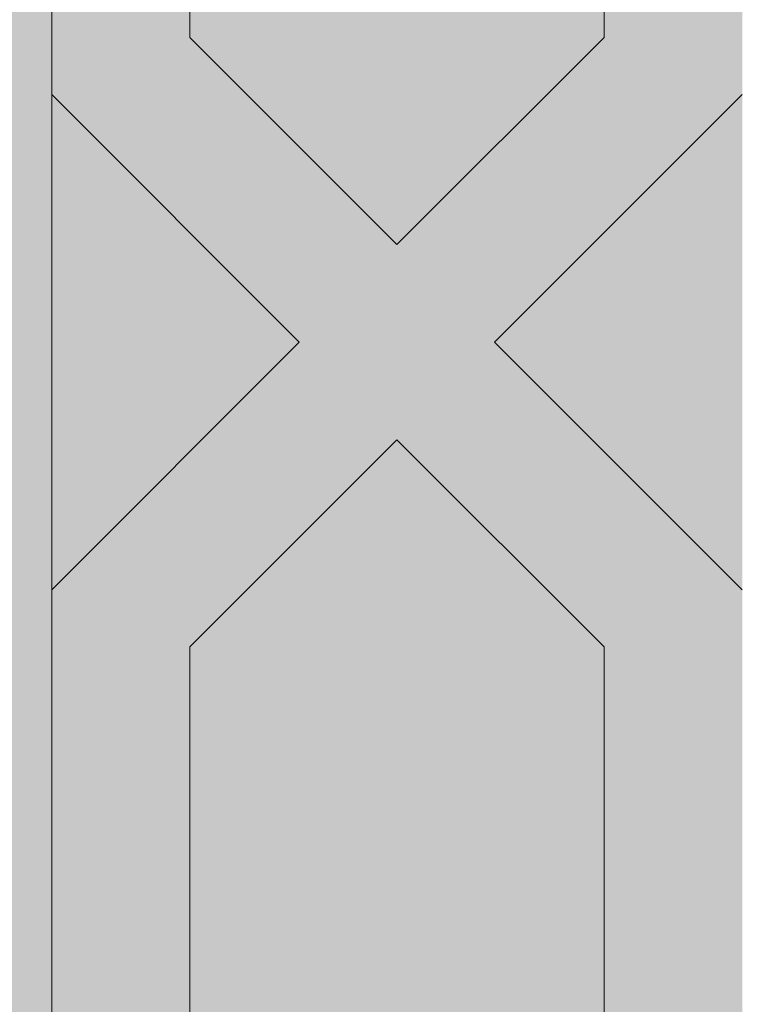
# Model space of a CAD drawing. Units: inches. Extents: x 844 to 2234, y 346 to 1084.
# Tile 17 of 93: x 1116.421 to 1117.756, y 703.242 to 705.06. Entities that reach past the tile are written whole.
import ezdxf

# ---------------------------------------------------------------- set-up
doc = ezdxf.new("R2010")
doc.units = ezdxf.units.IN
doc.header["$MEASUREMENT"] = 0
for name, color, linetype, lineweight in [('A-ANNO-DIMS', 2, 'Continuous', 18), ('furniture', 8, 'Continuous', 18), ('RA-AP-01$0$INT', 35, 'Continuous', 5)]:
    doc.layers.add(name, color=color, linetype=linetype, lineweight=lineweight)
doc.layers.add('RA-AP-01$0$FURN', color=3, linetype='Continuous')
doc.styles.get("Standard").update_dxf_attribs({"font": 'arial.ttf'})
doc.dimstyles.get("Standard").update_dxf_attribs({"dimtxt": 6, "dimasz": 3, "dimexe": 0.18, "dimexo": 0.0625, "dimgap": 0.09, "dimtad": 0, "dimtih": 1, "dimtoh": 1, "dimdec": 1, "dimzin": 0, "dimdsep": 46, "dimlunit": 3, "dimtxsty": 'Standard', "dimblk": 'ARCHTICK', "dimcen": 0.09, "dimadec": 0, "dimazin": 0, "dimtfac": 1, "dimtdec": 1, "dimtofl": 0, "dimtmove": 0, "dimatfit": 3, "dimfxl": 1, "dimtolj": 1, "dimtzin": 0, "dimarcsym": 0})

# ---------------------------------------------------------------- blocks, each defined once
blk = doc.blocks.new('A$C18D01794')
at = {"layer": 'RA-AP-01$0$INT'}
h = blk.add_hatch(color=256, dxfattribs=at)
h.paths.add_polyline_path([(4.355206456958071, -6.156712009588037), (4.355206456958071, -8.056712009588038), (5.455206456958072, -8.056712009588038), (5.455206456958072, -6.156712009588037)])
h.paths.add_polyline_path([(4.405206456958072, -8.006712009588039), (4.405206456958072, -6.206712009588038), (5.405206456958072, -6.206712009588038), (5.405206456958072, -8.006712009588039)], flags=16)
h = blk.add_hatch(color=256, dxfattribs=at)
h.paths.add_polyline_path([(4.505206456958071, -7.585498806127123), (4.46934859260189, -7.549640941759413), (4.505206456958071, -7.513783077414768), (4.505206456958071, -7.381963272220687), (4.469348592616735, -7.346105407867824), (4.505206456958071, -7.310247543514964), (4.505206456958071, -7.178427738324996), (4.469348592586679, -7.142569873965138), (4.505206456952245, -7.106712009588038), (4.476922185709333, -7.106712009588038), (4.455206456960671, -7.128427738343681), (4.433490728198047, -7.106712009588038), (4.405206456946033, -7.106712009588036), (4.441064321339216, -7.142569873969684), (4.40520645695807, -7.178427738362358), (4.405206456958072, -7.310247543472698), (4.441064321364728, -7.346105407867826), (4.40520645695807, -7.381963272262947), (4.40520645695807, -7.513783077378263), (4.441064321354429, -7.549640941786153), (4.405206456958072, -7.585498806170974), (4.405206456958072, -7.717318611286652), (4.441064321333084, -7.753176475673194), (4.405206456958072, -7.789034340036673), (4.405206456958072, -8.006712009588039), (4.644348592588106, -8.006712009588039), (4.680206456964639, -7.970854145211967), (4.716064321341165, -8.006712009588039), (4.869348592586113, -8.006712009588039), (4.905206456964143, -7.970854145210465), (4.941064321342174, -8.006712009588039), (5.094348592587118, -8.006712009588037), (5.130206456963649, -7.970854145211967), (5.166064321340178, -8.006712009588039), (5.405206456958072, -8.006712009588039), (5.405206456958072, -7.789034340024526), (5.369348592595202, -7.753176475673196), (5.40520645695807, -7.717318611298797), (5.40520645695807, -7.585498806158829), (5.369348592573859, -7.549640941786151), (5.40520645695807, -7.51378307739041), (5.40520645695807, -7.381963272250803), (5.36934859256356, -7.346105407867824), (5.405206456958072, -7.310247543484846), (5.405206456958072, -7.178427738350217), (5.369348592589068, -7.142569873969682), (5.405206456982249, -7.106712009588038), (5.376922185730244, -7.106712009588038), (5.355206456967613, -7.128427738343679), (5.333490728218955, -7.10671200958804), (5.305206456976043, -7.106712009588042), (5.341064321341609, -7.142569873965136), (5.305206456958072, -7.178427738337141), (5.305206456958072, -7.310247543502816), (5.34106432131155, -7.346105407867824), (5.305206456958072, -7.381963272232832), (5.30520645695807, -7.513783077402624), (5.341064321326395, -7.549640941759413), (5.305206456958072, -7.585498806139263), (5.305206456958072, -7.717318611299605), (5.341064321347738, -7.753176475677737), (5.305206456958072, -7.78903434007894), (5.30520645695807, -7.906712009588039), (5.166064321336834, -7.906712009588039), (5.130206456963647, -7.942569873961684), (5.094348592590464, -7.906712009588039), (4.941064321338827, -7.906712009588041), (4.905206456964145, -7.942569873963183), (4.869348592589459, -7.906712009588039), (4.716064321337822, -7.906712009588041), (4.680206456964641, -7.942569873961684), (4.644348592591453, -7.906712009588039), (4.505206456958071, -7.906712009588039), (4.505206456958071, -7.789034340066795), (4.469348592580545, -7.753176475677738), (4.505206456958071, -7.717318611311748)])
h.paths.add_polyline_path([(4.485206456974132, -7.709034340046354), (4.45520645695909, -7.739034340051736), (4.425206456974128, -7.709034340057131), (4.425206456993394, -7.593783077384998), (4.45520645699153, -7.563783077396511), (4.485206456993396, -7.593783077408017)], flags=16)
h.paths.add_polyline_path([(4.455206456954537, -7.767318611299197), (4.485206456958242, -7.797318611312542), (4.48520645695951, -7.912569873958716), (4.45520645695415, -7.942569873954422), (4.425206456957888, -7.912569873967813), (4.425206456957888, -7.797318611286197)], flags=16)
h.paths.add_polyline_path([(4.455206456964794, -7.535498806149051), (4.42520645696469, -7.5054988061393), (4.425206456983954, -7.390247543486406), (4.455206456990734, -7.360247543489279), (4.485206456983953, -7.39024754349214), (4.485206456964687, -7.505498806158811)], flags=16)
h.paths.add_polyline_path([(4.499348592588947, -7.926712009585049), (4.636064321340932, -7.926712009585049), (4.666064321342317, -7.956712009586821), (4.636064321343707, -7.986712009585048), (4.499348592575121, -7.986712009585048), (4.469348592591685, -7.956712009591957)], flags=16)
h.paths.add_polyline_path([(4.425206456957888, -7.940854145195974), (4.471064321332215, -7.986712009585049), (4.425206456957888, -7.986712009585049)], flags=16)
h.paths.add_polyline_path([(4.455206456990734, -7.331963272246367), (4.425206456989053, -7.301963272254337), (4.425206456969784, -7.186712009596224), (4.455206456965226, -7.156712009591144), (4.485206456969787, -7.186712009586051), (4.485206456989053, -7.301963272238404)], flags=16)
h.paths.add_polyline_path([(4.72434859258714, -7.926712009586255), (4.861064321340141, -7.926712009586248), (4.891064321340324, -7.956712009586823), (4.861064321340513, -7.986712009586252), (4.724348592586768, -7.986712009586252), (4.694348592586956, -7.956712009586821)], flags=16)
h.paths.add_polyline_path([(4.919348592587961, -7.956712009586821), (4.949348592588145, -7.92671200958625), (5.08606432134115, -7.926712009586253), (5.116064321341327, -7.956712009586823), (5.086064321341519, -7.986712009586252), (4.949348592587774, -7.986712009586252)], flags=16)
h.paths.add_polyline_path([(5.144348592585967, -7.956712009586823), (5.174348592587358, -7.926712009585049), (5.311064321339338, -7.926712009585049), (5.3410643213366, -7.956712009591957), (5.311064321353163, -7.986712009585048), (5.174348592584576, -7.986712009585048)], flags=16)
h.paths.add_polyline_path([(5.32520645693489, -7.593783077408021), (5.355206456936755, -7.563783077396511), (5.385206456934894, -7.593783077384998), (5.38520645695416, -7.709034340057128), (5.355206456969194, -7.739034340051736), (5.325206456954153, -7.709034340046352)], flags=16)
h.paths.add_polyline_path([(5.325206456970042, -7.797318611312542), (5.355206456973747, -7.767318611299197), (5.385206456970398, -7.7973186112862), (5.385206456970398, -7.912569873967816), (5.355206456974136, -7.942569873954422), (5.325206456968778, -7.912569873958716)], flags=16)
h.paths.add_polyline_path([(5.325206456963599, -7.505498806158811), (5.325206456944333, -7.39024754349214), (5.355206456937552, -7.360247543489279), (5.385206456944332, -7.39024754348641), (5.385206456963596, -7.505498806139303), (5.355206456963492, -7.53549880614905)], flags=16)
h.paths.add_polyline_path([(5.32520645693923, -7.301963272238403), (5.3252064569585, -7.186712009586051), (5.355206456963062, -7.156712009591142), (5.3852064569585, -7.186712009596224), (5.385206456939234, -7.301963272254338), (5.355206456937552, -7.331963272246369)], flags=16)
h.paths.add_polyline_path([(5.339348592596071, -7.986712009585048), (5.385206456970398, -7.940854145195972), (5.385206456970396, -7.986712009585048)], flags=16)
h = blk.add_hatch(color=256, dxfattribs=at)
h.paths.add_polyline_path([(4.469348592586677, -7.142569873965136), (4.505206456958073, -7.178427738324996), (4.505206456958071, -7.106712009582215)])
h.paths.add_polyline_path([(4.455206456960671, -7.128427738343681), (4.476922185709333, -7.106712009588038), (4.433490728198045, -7.106712009588038)])
h.paths.add_polyline_path([(4.405206456958073, -7.178427738362358), (4.441064321339218, -7.142569873969684), (4.40520645695807, -7.106712009600073)])
h.paths.add_polyline_path([(4.425206456989053, -7.301963272254335), (4.455206456990736, -7.331963272246371), (4.485206456989055, -7.301963272238399), (4.48520645696979, -7.186712009586054), (4.455206456965227, -7.15671200959114), (4.425206456969784, -7.186712009596224)])
h.paths.add_polyline_path([(4.505206456958073, -7.381963272220689), (4.505206456958071, -7.310247543514961), (4.469348592616738, -7.346105407867826)])
h.paths.add_polyline_path([(4.425206456964688, -7.5054988061393), (4.455206456964794, -7.535498806149051), (4.485206456964689, -7.505498806158811), (4.485206456983951, -7.390247543492138), (4.455206456990736, -7.360247543489277), (4.425206456983956, -7.39024754348641)])
h.paths.add_polyline_path([(4.425206456974126, -7.709034340057128), (4.455206456959092, -7.739034340051736), (4.485206456974132, -7.709034340046356), (4.485206456993396, -7.593783077408017), (4.45520645699153, -7.563783077396511), (4.425206456993394, -7.593783077384999)])
h.paths.add_polyline_path([(4.46934859260189, -7.549640941759415), (4.505206456958071, -7.585498806127123), (4.505206456958073, -7.513783077414766)])
h.paths.add_polyline_path([(4.405206456958073, -7.585498806170972), (4.441064321354427, -7.549640941786151), (4.405206456958072, -7.513783077378263)])
h.paths.add_polyline_path([(4.405206456958072, -7.789034340036673), (4.441064321333084, -7.753176475673194), (4.405206456958072, -7.71731861128665)])
h.paths.add_polyline_path([(4.469348592580547, -7.75317647567774), (4.505206456958071, -7.789034340066795), (4.505206456958071, -7.717318611311744)])
h.paths.add_polyline_path([(4.425206456957888, -7.912569873967814), (4.45520645695415, -7.942569873954422), (4.485206456959507, -7.912569873958718), (4.48520645695824, -7.797318611312542), (4.455206456954537, -7.767318611299197), (4.425206456957888, -7.797318611286202)])
h.paths.add_polyline_path([(4.425206456957888, -7.986712009585049), (4.471064321332215, -7.986712009585049), (4.425206456957888, -7.940854145195972)])
h.paths.add_polyline_path([(4.499348592575121, -7.986712009585048), (4.636064321343707, -7.986712009585049), (4.666064321342317, -7.956712009586823), (4.636064321340932, -7.926712009585049), (4.499348592588945, -7.926712009585049), (4.469348592591685, -7.95671200959196)])
h.paths.add_polyline_path([(4.680206456964641, -7.942569873961684), (4.716064321337824, -7.906712009588039), (4.644348592591454, -7.906712009588039)])
h.paths.add_polyline_path([(4.644348592588108, -8.006712009588039), (4.716064321341167, -8.006712009588039), (4.680206456964637, -7.970854145211964)])
h.paths.add_polyline_path([(4.724348592586768, -7.98671200958625), (4.861064321340514, -7.986712009586252), (4.891064321340324, -7.956712009586819), (4.861064321340141, -7.92671200958625), (4.724348592587134, -7.926712009586255), (4.694348592586957, -7.956712009586821)])
h.paths.add_polyline_path([(4.905206456964143, -7.942569873963183), (4.941064321338827, -7.906712009588039), (4.869348592589457, -7.906712009588037)])
h.paths.add_polyline_path([(4.869348592586113, -8.006712009588039), (4.941064321342172, -8.006712009588037), (4.905206456964145, -7.970854145210463)])
h.paths.add_polyline_path([(4.949348592587774, -7.986712009586252), (5.086064321341521, -7.986712009586252), (5.116064321341329, -7.956712009586823), (5.08606432134115, -7.926712009586253), (4.949348592588145, -7.92671200958625), (4.919348592587961, -7.956712009586819)])
h.paths.add_polyline_path([(5.130206456963645, -7.942569873961684), (5.166064321336834, -7.906712009588039), (5.094348592590464, -7.906712009588039)])
h.paths.add_polyline_path([(5.094348592587119, -8.006712009588039), (5.166064321340178, -8.006712009588039), (5.130206456963651, -7.970854145211967)])
h.paths.add_polyline_path([(5.174348592584578, -7.986712009585048), (5.311064321353163, -7.986712009585048), (5.341064321336602, -7.956712009591958), (5.31106432133934, -7.926712009585049), (5.174348592587352, -7.926712009585049), (5.144348592585969, -7.956712009586823)])
h.paths.add_polyline_path([(5.325206456968778, -7.912569873958718), (5.355206456974136, -7.942569873954422), (5.385206456970396, -7.912569873967814), (5.385206456970396, -7.797318611286199), (5.355206456973747, -7.767318611299197), (5.325206456970044, -7.797318611312544)])
h.paths.add_polyline_path([(5.339348592596073, -7.986712009585048), (5.385206456970396, -7.986712009585049), (5.385206456970398, -7.94085414519597)])
h.paths.add_polyline_path([(5.325206456954155, -7.709034340046354), (5.355206456969194, -7.739034340051734), (5.38520645695416, -7.709034340057128), (5.385206456934896, -7.593783077384999), (5.355206456936758, -7.563783077396513), (5.325206456934888, -7.593783077408019)])
h.paths.add_polyline_path([(5.305206456958072, -7.789034340078938), (5.341064321347739, -7.753176475677738), (5.305206456958072, -7.717318611299605)])
h.paths.add_polyline_path([(5.369348592595204, -7.753176475673194), (5.40520645695807, -7.789034340024526), (5.405206456958072, -7.717318611298798)])
h.paths.add_polyline_path([(5.405206456958072, -7.585498806158831), (5.405206456958072, -7.513783077390407), (5.369348592573857, -7.549640941786151)])
h.paths.add_polyline_path([(5.305206456958072, -7.585498806139266), (5.341064321326393, -7.549640941759413), (5.305206456958072, -7.513783077402626)])
h.paths.add_polyline_path([(5.325206456963599, -7.50549880615881), (5.355206456963494, -7.535498806149055), (5.385206456963598, -7.505498806139302), (5.385206456944334, -7.390247543486411), (5.355206456937552, -7.360247543489279), (5.325206456944333, -7.39024754349214)])
h.paths.add_polyline_path([(5.305206456958072, -7.38196327223283), (5.341064321311551, -7.346105407867824), (5.305206456958072, -7.31024754350282)])
h.paths.add_polyline_path([(5.325206456939231, -7.301963272238404), (5.355206456937552, -7.331963272246369), (5.385206456939235, -7.301963272254335), (5.385206456958502, -7.186712009596224), (5.355206456963061, -7.156712009591142), (5.3252064569585, -7.186712009586051)])
h.paths.add_polyline_path([(5.404581768715993, -7.381338584008926, -0.001217816984214), (5.405206456958072, -7.381112009582329), (5.405206456958072, -7.310247543484846), (5.369348592563558, -7.346105407867826)])
h.paths.add_polyline_path([(5.36934859258907, -7.142569873969684), (5.40520645695807, -7.178427738350215), (5.405206456958072, -7.106712009612218)])
h.paths.add_polyline_path([(5.355206456967613, -7.128427738343683), (5.376922185730239, -7.106712009588038), (5.333490728218953, -7.10671200958804)])
h.paths.add_polyline_path([(5.30520645695807, -7.178427738337139), (5.341064321341609, -7.142569873965134), (5.305206456958074, -7.10671200957007)])
for p, q in [((4.425206456993394, -7.593783077384996), (4.425206456974128, -7.709034340057129)), ((4.485206456993396, -7.593783077408017), (4.485206456974132, -7.709034340046354)), ((4.425206456974128, -7.709034340057129), (4.455206456959092, -7.739034340051736)), ((4.485206456974132, -7.709034340046354), (4.455206456959092, -7.739034340051736)), ((4.405206456963013, -7.717318611291593), (4.441064321333084, -7.753176475673194)), ((4.505206456963013, -7.717318611306806), (4.469348592580547, -7.753176475677738)), ((4.441064321333084, -7.753176475673194), (4.405206456950156, -7.789034340044587)), ((4.469348592580547, -7.753176475677738), (4.505206456951941, -7.789034340060664)), ((4.455206456954537, -7.767318611299197), (4.425206456957888, -7.797318611286199)), ((4.455206456954537, -7.767318611299197), (4.485206456958242, -7.797318611312544)), ((4.425206456957888, -7.797318611286199), (4.425206456957888, -7.912569873967814)), ((4.485206456959509, -7.912569873958718), (4.485206456958242, -7.797318611312544))]:
    blk.add_line(p, q, dxfattribs=at)
blk.add_lwpolyline([(5.405206456958072, -8.006712009588039), (4.405206456958072, -8.006712009588039), (4.405206456958072, -7.106712009588038)], dxfattribs=at)
blk = doc.blocks.new('A$C5D2F253E')
at = {"layer": 'RA-AP-01$0$FURN', "xscale": -0.7999999999883585, "yscale": 0.7999999999883585, "zscale": 0.8, "rotation": 90}
blk.add_blockref('A$C18D01794', (-5.687757199772477, 4.75791982714071), dxfattribs=at)
blk = doc.blocks.new('_ArchTick')
at = {"color": 0, "linetype": 'ByBlock', "const_width": 0.15}
blk.add_lwpolyline([(-0.5, -0.5), (0.5, 0.5)], dxfattribs=at)
blk = doc.blocks.new('*D144')
at = {"layer": 'A-ANNO-DIMS', "color": 0, "lineweight": -2, "transparency": 16777216}
for p, q in [((1096.615948, 439.3732739999999), (1096.615948, 1074.743301)), ((1143.115948, 492.373274), (1143.115948, 1074.743301)), ((1096.615948, 1074.563301), (1102.481950728513, 1074.563301)), ((1143.115948, 1074.563301), (1137.249945271487, 1074.563301))]:
    blk.add_line(p, q, dxfattribs=at)
at = {"layer": 'Defpoints', "color": 0, "transparency": 16777216}
for p in [(1143.115948, 1074.563301), (1143.115948, 492.3107739999999), (1096.615948, 439.3107739999999)]:
    blk.add_point(p, dxfattribs=at)
at = {"layer": 'A-ANNO-DIMS', "color": 0, "lineweight": -2, "transparency": 16777216, "xscale": 3, "yscale": 3, "zscale": 3, "rotation": 180}
blk.add_blockref('_ArchTick', (1096.615948, 1074.563301), dxfattribs=at)
at = {"layer": 'A-ANNO-DIMS', "color": 0, "lineweight": -2, "transparency": 16777216, "xscale": 3, "yscale": 3, "zscale": 3}
blk.add_blockref('_ArchTick', (1143.115948, 1074.563301), dxfattribs=at)
at = {"layer": 'A-ANNO-DIMS', "color": 0, "transparency": 16777216, "insert": (1119.865948, 1074.563301), "char_height": 6, "attachment_point": 5}
blk.add_mtext('\\A1;3\'-10 1/2"', dxfattribs=at)

msp = doc.modelspace()

# ---------------------------------------------------------------- block references
at = {"layer": 'furniture', "xscale": 15.94108302203742, "yscale": 15.94108302203742, "zscale": 15.94108302203742, "rotation": 90}
msp.add_blockref('A$C5D2F253E', (1136.147844094663, 696.2584716700112), dxfattribs=at)

# ---------------------------------------------------------------- dimensions: what is measured, and where the dimension line sits
at = {"layer": 'A-ANNO-DIMS'}
dim = msp.add_linear_dim(base=(1143.115948, 1074.563301), p1=(1096.615948, 439.3107739999999), p2=(1143.115948, 492.3107739999999), dimstyle='Standard', override={"dimdec": 1, "dimlfac": 1, "dimrnd": 0, "dimzin": 1, "dimdsep": 46, "dimlunit": 4, "dimfrac": 2}, dxfattribs=at)
dim.commit()
dim.dimension.update_dxf_attribs({"geometry": '*D144', "text_midpoint": (1119.865948, 1074.563301)})

doc.saveas('drawing.dxf')
